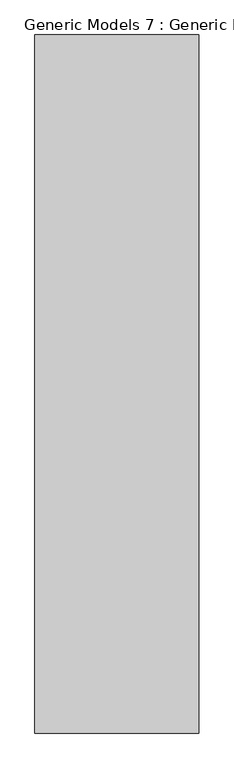
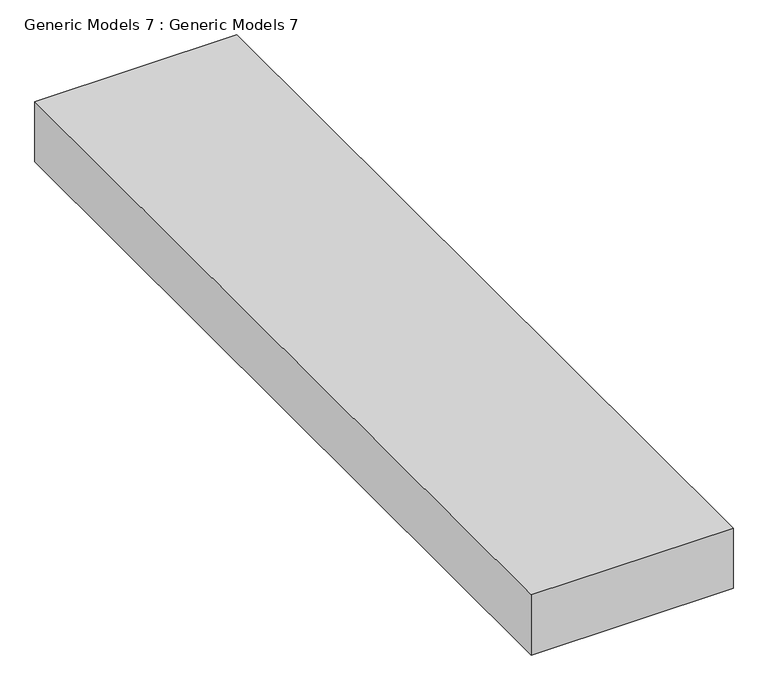
"""IFC4 building model written with IfcOpenShell, lengths in millimetres: proxy geometry, Generic Models 7 : Generic Models 7."""

from ifc_helpers import new_model, si_unit, frame, origin, place, context, project, spatial, polyline, outline, extrude, source, transform, mapped, element, save


def generic_models_7_generic_models_7_8d3c1b96(model_context):
    return source(origin(), model_context, "Body", "SweptSolid", [
        extrude(outline(polyline([(-3319.1999834, -2669.7777232), (-3319.1999834, -4728.6561255), (-3802.4859258, -4728.6561255), (-3802.4859258, -2669.7777232), (-3319.1999834, -2669.7777232)])), frame((0.0, 0.0, 2487.6320874), z_axis=(0.0, 0.0, 1.0), x_axis=(1.0, 0.0, 0.0)), (0.0, 0.0, 1.0), 152.4),
    ])


if __name__ == "__main__":
    model = new_model("IFC4")
    model_context = context("Model", 3, world=origin())
    ifc_project = project(units=[si_unit("LENGTHUNIT", "METRE", prefix="MILLI")], contexts=[model_context])
    site = spatial("IfcSite", under=ifc_project)
    building = spatial("IfcBuilding", under=site)
    placement = place(None, origin())
    generic_models_7_generic_models_7_shape = generic_models_7_generic_models_7_8d3c1b96(model_context)
    element("IfcBuildingElementProxy", 1, Name="Generic Models 7 : Generic Models 7", ObjectType="Generic Models 7 : Generic Models 7", at=placement, inside=building, context=model_context, shape_type="MappedRepresentation", body=[
        mapped(generic_models_7_generic_models_7_shape, transform((0.0, 0.0, 0.0), x_axis=(1.0, 0.0, 0.0), y_axis=(0.0, 1.0, 0.0), z_axis=(0.0, 0.0, 1.0))),
    ])
    save(model, "model.ifc")
